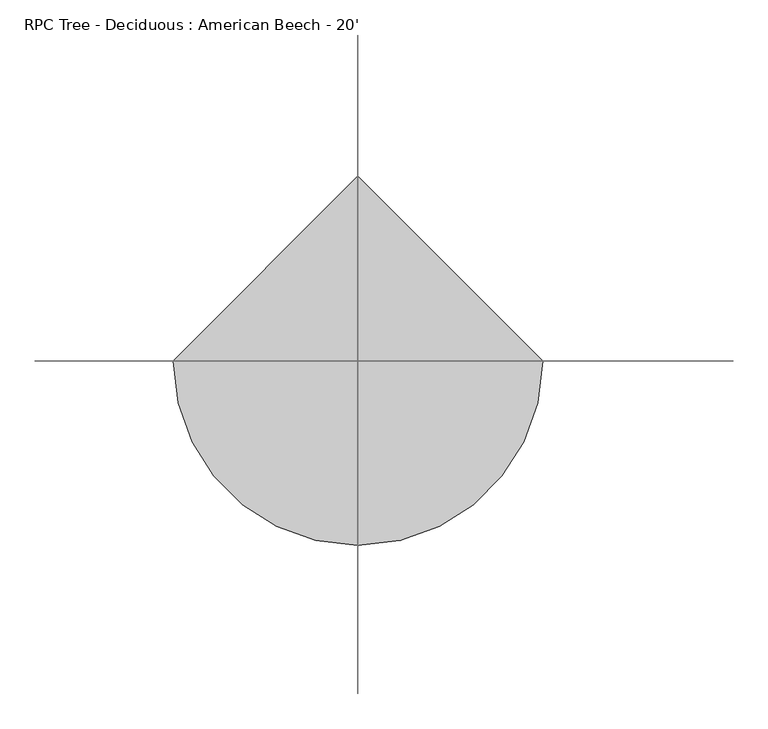
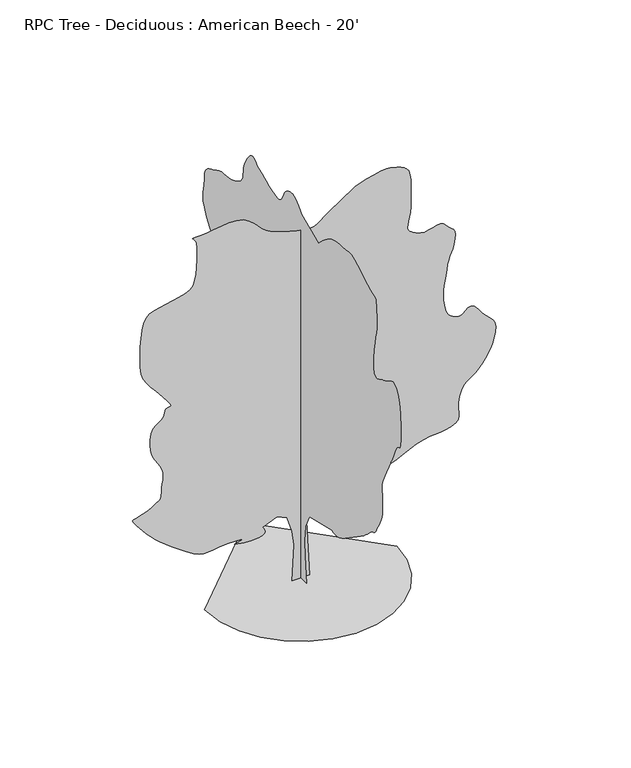
"""IFC4 building model written with IfcOpenShell, lengths in millimetres: geographic element geometry, RPC Tree - Deciduous : American Beech - 20'."""

from ifc_helpers import new_model, si_unit, origin, place, context, project, spatial, triangles, source, transform, mapped, element, save


def rpc_tree_deciduous_american_beech_20_b3c041c8(model_context):
    return source(origin(), model_context, "Body", "Tessellation", [
        triangles([(0.0009889, 136.856581, 0.0), (0.0009889, -149.8547884, 0.0), (0.0009889, -111.6264895, 420.510052), (0.0009889, -102.0697236, 659.4353302), (0.0009889, -121.1832463, 898.3606447), (0.0009889, -235.8678885, 1118.172373), (0.0009889, -818.8458761, 1261.5275036), (0.0009889, -849.9431059, 1249.7139805), (0.0009889, -883.2933231, 1240.7427258), (0.0009889, -921.1596891, 1237.4533916), (0.0009889, -965.7976622, 1242.6934788), (0.0009889, -1019.4603024, 1259.3000233), (0.0009889, -1084.4081549, 1290.1152935), (0.0009889, -1162.8992941, 1337.984174), (0.0009889, -1478.2811337, 1557.7959023), (0.0009889, -1522.8632961, 1589.1420994), (0.0009889, -1566.942437, 1618.9819931), (0.0009889, -1611.1893002, 1649.3249084), (0.0009889, -1656.2718681, 1682.1772636), (0.0009889, -1702.8579781, 1719.5406807), (0.0009889, -1751.6183739, 1763.4243393), (0.0009889, -1803.2210381, 1815.834803), (0.0009889, -1847.9404015, 1858.0191467), (0.0009889, -1878.9512993, 1877.1351311), (0.0009889, -1901.2702858, 1884.0440117), (0.0009889, -1919.9112991, 1889.616782), (0.0009889, -1939.8884228, 1904.7196392), (0.0009889, -1966.2180656, 1940.2161644), (0.0009889, -2003.916782, 2006.9774963), (0.0009889, -2044.9607883, 2083.2080177), (0.0009889, -2078.313549, 2145.2324295), (0.0009889, -2104.4754696, 2201.0692829), (0.0009889, -2123.9521877, 2258.7475937), (0.0009889, -2137.244109, 2326.2862038), (0.0009889, -2144.8488773, 2411.7141289), (0.0009889, -2147.2746014, 2523.0550072), (0.0009889, -2142.5373905, 2624.8889076), (0.0009889, -2132.7863869, 2688.2873634), (0.0009889, -2124.7040314, 2730.9338882), (0.0009889, -2124.9835201, 2770.583503), (0.0009889, -2140.3072941, 2824.9394875), (0.0009889, -2177.3659332, 2911.7568626), (0.0009889, -2242.84464, 3048.6883301), (0.0009889, -2308.7119858, 3181.9621719), (0.0009889, -2348.5011269, 3259.3812836), (0.0009889, -2371.2366577, 3301.215358), (0.0009889, -2385.9484051, 3327.6567673), (0.0009889, -2401.6632889, 3358.9496246), (0.0009889, -2427.4088104, 3415.3121727), (0.0009889, -2472.2118896, 3516.9885246), (0.0009889, -2522.8114174, 3609.6476944), (0.0009889, -2561.0332123, 3645.1568642), (0.0009889, -2588.5669968, 3652.9040657), (0.0009889, -2607.0580193, 3662.3273277), (0.0009889, -2618.2087921, 3702.8402618), (0.0009889, -2623.669796, 3803.856189), (0.0009889, -2625.117382, 3994.8390083), (0.0009889, -2615.3639076, 4210.713913), (0.0009889, -2589.2271309, 4371.4450905), (0.0009889, -2551.406765, 4483.8402649), (0.0009889, -2506.5400269, 4554.7824463), (0.0009889, -2459.3391289, 4591.1043571), (0.0009889, -2414.4802391, 4599.6895889), (0.0009889, -2376.641851, 4587.3705734), (0.0009889, -2343.8477772, 4566.9491455), (0.0009889, -2310.8862717, 4546.8576393), (0.0009889, -2277.5893215, 4527.4521378), (0.0009889, -2243.7921112, 4509.0116936), (0.0009889, -2209.3243023, 4491.9426773), (0.0009889, -2174.0232594, 4476.5250137), (0.0009889, -2137.7164639, 4463.1392029), (0.0009889, -2096.4236355, 4443.6572525), (0.0009889, -2049.6139927, 4418.4858238), (0.0009889, -2002.3013283, 4400.6805153), (0.0009889, -1959.504958, 4403.2713455), (0.0009889, -1926.2359131, 4439.313913), (0.0009889, -1907.5110386, 4521.8132378), (0.0009889, -1908.3467434, 4663.8246277), (0.0009889, -1923.6450829, 4819.4253044), (0.0009889, -1942.954224, 4940.7356323), (0.0009889, -1963.266647, 5037.9669067), (0.0009889, -1981.572361, 5121.3298416), (0.0009889, -1994.8642822, 5201.0354416), (0.0009889, -2000.1296585, 5287.2429703), (0.0009889, -1994.3614059, 5390.1634323), (0.0009889, -1986.3653824, 5488.9190323), (0.0009889, -1983.048143, 5559.911792), (0.0009889, -1978.5625156, 5609.3407516), (0.0009889, -1967.0562412, 5643.3764648), (0.0009889, -1942.6748806, 5668.2429703), (0.0009889, -1899.5709709, 5690.0869858), (0.0009889, -1831.8926891, 5715.1063889), (0.0009889, -1748.4408062, 5751.9616974), (0.0009889, -1662.820015, 5800.5261749), (0.0009889, -1576.3582867, 5853.7903656), (0.0009889, -1490.4020508, 5904.6919098), (0.0009889, -1406.2848015, 5946.2207703), (0.0009889, -1325.3426491, 5971.3924896), (0.0009889, -1248.913884, 5973.1447083), (0.0009889, -1174.2403896, 5963.3406555), (0.0009889, -1098.5636135, 5956.711409), (0.0009889, -1023.222064, 5950.5641098), (0.0009889, -949.5518515, 5942.2588028), (0.0009889, -878.8914843, 5929.1264648), (0.0009889, -812.5771454, 5908.4509827), (0.0009889, -751.9472706, 5877.5644958), (0.0009889, -697.9494038, 5841.2678741), (0.0009889, -649.9687569, 5805.9618896), (0.0009889, -607.0045916, 5771.4942261), (0.0009889, -568.0511189, 5737.7119858), (0.0009889, -532.1075644, 5704.4128555), (0.0009889, -498.1706097, 5671.4433563), (0.0009889, -465.2369368, 5638.6523346), (0.0009889, -16.056217, 5829.7871796), (0.0009889, 22.8405617, 5872.4339951), (0.0009889, 61.6537222, 5913.023378), (0.0009889, 100.2998553, 5949.3961578), (0.0009889, 138.6950317, 5979.5204819), (0.0009889, 176.7559443, 6001.2883392), (0.0009889, 214.3990318, 6012.5911377), (0.0009889, 251.5404602, 6011.3720261), (0.0009889, 287.2056524, 6002.4312927), (0.0009889, 320.3628219, 5991.305809), (0.0009889, 350.8454089, 5977.0055191), (0.0009889, 378.4856913, 5958.5397858), (0.0009889, 403.1160919, 5934.892392), (0.0009889, 424.5689612, 5905.047702), (0.0009889, 442.6817001, 5868.0144974), (0.0009889, 459.9562634, 5826.9425858), (0.0009889, 480.2407084, 5787.547316), (0.0009889, 505.3740581, 5752.6727005), (0.0009889, 537.1926464, 5725.138916), (0.0009889, 577.5380399, 5707.7911377), (0.0009889, 628.2491524, 5703.5239563), (0.0009889, 691.1650068, 5715.1063889), (0.0009889, 759.6790661, 5736.9754028), (0.0009889, 826.1890326, 5761.3593796), (0.0009889, 891.0251186, 5787.8263687), (0.0009889, 954.5251671, 5815.9694183), (0.0009889, 1017.0218611, 5845.3577408), (0.0009889, 1078.8506453, 5875.5832214), (0.0009889, 1140.3440575, 5906.2412338), (0.0009889, 1169.0715191, 5932.3524307), (0.0009889, 1198.1316639, 5955.3649796), (0.0009889, 1227.8624073, 5972.2052307), (0.0009889, 1258.5938164, 5979.7489563), (0.0009889, 1290.6664227, 5974.9230881), (0.0009889, 1324.4078224, 5954.6539764), (0.0009889, 1360.1557858, 5915.7918137), (0.0009889, 1395.1799561, 5868.217392), (0.0009889, 1426.1908539, 5822.9544571), (0.0009889, 1452.6880737, 5778.8856354), (0.0009889, 1474.1715008, 5734.7912338), (0.0009889, 1490.1379681, 5689.5538788), (0.0009889, 1500.0845993, 5641.9538773), (0.0009889, 1503.510989, 5590.8494385), (0.0009889, 1507.2168674, 5539.3380478), (0.0009889, 1519.1142517, 5491.1793594), (0.0009889, 1540.3740005, 5446.1704788), (0.0009889, 1572.1672634, 5404.1846695), (0.0009889, 1615.6596668, 5365.0428726), (0.0009889, 1672.0274471, 5328.5689362), (0.0009889, 1742.4363762, 5294.5832199), (0.0009889, 1817.5288857, 5269.1836075), (0.0009889, 1887.9378147, 5255.1373718), (0.0009889, 1954.8363476, 5247.4407486), (0.0009889, 2019.3956337, 5241.0911362), (0.0009889, 2082.7839157, 5231.0580276), (0.0009889, 2146.1721977, 5212.3382401), (0.0009889, 2210.7313385, 5179.9024292), (0.0009889, 2276.3498623, 5145.3580261), (0.0009889, 2340.1267834, 5118.8404587), (0.0009889, 2399.0573433, 5093.1356323), (0.0009889, 2450.1315514, 5061.106192), (0.0009889, 2490.3372368, 5015.5136261), (0.0009889, 2516.667025, 4949.193837), (0.0009889, 2526.1132507, 4854.9597633), (0.0009889, 2532.46577, 4758.008123), (0.0009889, 2546.5044479, 4681.9348595), (0.0009889, 2560.7285797, 4617.2411339), (0.0009889, 2567.5865913, 4554.3760757), (0.0009889, 2559.5600464, 4483.8402649), (0.0009889, 2529.1232414, 4396.0578323), (0.0009889, 2468.7702393, 4281.5543564), (0.0009889, 2394.0992157, 4166.6192207), (0.0009889, 2326.6139454, 4078.2525215), (0.0009889, 2267.6553349, 4007.9707649), (0.0009889, 2218.5596397, 3947.1884285), (0.0009889, 2180.6679119, 3887.4223091), (0.0009889, 2155.3111748, 3820.1377533), (0.0009889, 2143.8328056, 3736.8001076), (0.0009889, 2149.4334812, 3646.0204742), (0.0009889, 2171.0820145, 3561.7686401), (0.0009889, 2203.7667927, 3483.5112076), (0.0009889, 2242.4687908, 3410.790937), (0.0009889, 2282.1714546, 3343.1000107), (0.0009889, 2317.8662235, 3279.9047401), (0.0009889, 2344.5311657, 3220.7225967), (0.0009889, 2370.3577869, 3180.6921913), (0.0009889, 2402.5396889, 3164.8934464), (0.0009889, 2434.5538685, 3157.7813805), (0.0009889, 2459.8827003, 3143.8113029), (0.0009889, 2472.0037628, 3107.4638123), (0.0009889, 2464.3963783, 3033.1433487), (0.0009889, 2430.5432121, 2905.3305107), (0.0009889, 2383.9011463, 2761.3378464), (0.0009889, 2340.6017544, 2643.9136185), (0.0009889, 2298.1379219, 2545.7425758), (0.0009889, 2254.0028252, 2459.415287), (0.0009889, 2205.6894951, 2377.6095245), (0.0009889, 2150.6857304, 2292.9614937), (0.0009889, 2086.4897942, 2198.1177189), (0.0009889, 2022.098085, 2102.5196297), (0.0009889, 1968.0723129, 2019.6267242), (0.0009889, 1924.2446102, 1948.102747), (0.0009889, 1890.4447838, 1886.6067913), (0.0009889, 1866.5103436, 1833.8078339), (0.0009889, 1852.2735672, 1788.3620613), (0.0009889, 1847.564407, 1748.9361248), (0.0009889, 1851.5776794, 1721.8800728), (0.0009889, 1860.940044, 1709.2029396), (0.0009889, 1871.6386642, 1703.0459026), (0.0009889, 1879.6624477, 1695.5504299), (0.0009889, 1881.0010288, 1678.8600243), (0.0009889, 1871.6386642, 1645.1186245), (0.0009889, 1847.564407, 1586.4675533), (0.0009889, 1827.5314728, 1524.5828133), (0.0009889, 1825.3850922, 1482.2587978), (0.0009889, 1829.7590984, 1453.3104195), (0.0009889, 1829.2865982, 1431.547649), (0.0009889, 1812.5961926, 1410.7907764), (0.0009889, 1768.3214241, 1384.8497726), (0.0009889, 1685.0958355, 1347.5421661), (0.0009889, 1594.399918, 1309.4244347), (0.0009889, 1528.281134, 1282.5080544), (0.0009889, 1476.2059696, 1262.7823689), (0.0009889, 1427.6412014, 1246.2316349), (0.0009889, 1372.05317, 1228.8453415), (0.0009889, 1298.9138844, 1206.6102161), (0.0009889, 1197.6871416, 1175.5154572), (0.0009889, 1096.069289, 1145.7009253), (0.0009889, 1022.5387482, 1127.7557997), (0.0009889, 967.7331545, 1118.3400227), (0.0009889, 922.2874546, 1114.10329), (0.0009889, 876.8442255, 1111.7080873), (0.0009889, 822.0360884, 1107.806654), (0.0009889, 748.5055475, 1099.0588594), (0.0009889, 662.4935011, 1085.0990284), (0.0009889, 576.4788749, 1068.1292793), (0.0009889, 490.4667558, 1048.6551046), (0.0009889, 404.4521296, 1027.1717503), (0.0009889, 318.4400468, 1004.1847086), (0.0009889, 232.4266923, 980.1943851), (0.0009889, 146.4133378, 955.7037289), (136.1842383, 0.0003154, 0.014068), (-131.4120823, 0.0003154, 0.014068), (-102.7410489, 0.0002819, 563.8778998), (-131.4120823, 0.0002692, 793.2477293), (-207.8684348, 0.0002549, 1032.1729712), (-360.7819027, 0.0002501, 1108.6296415), (-580.5936673, 0.0002549, 1013.0594576), (-562.704425, 0.0002564, 988.5662579), (-548.0765751, 0.000258, 964.5784779), (-539.9688578, 0.0002596, 941.5914362), (-541.6401947, 0.0002612, 920.1080818), (-556.3518694, 0.0002628, 900.6313637), (-587.3627672, 0.0002628, 883.6641581), (-637.9342443, 0.0002644, 869.704327), (-697.421093, 0.0002644, 860.4815615), (-753.4001616, 0.0002644, 856.775683), (-806.4506298, 0.0002644, 857.667271), (-857.1617786, 0.0002644, 862.2366869), (-906.117802, 0.0002644, 869.5645826), (-953.9028214, 0.0002628, 878.731465), (-1001.1011759, 0.0002628, 888.8178406), (-953.2881786, 0.0002628, 900.9945683), (-913.501581, 0.0002612, 912.5008427), (-889.7601522, 0.0002612, 922.6710068), (-890.0954515, 0.0002596, 930.8345346), (-922.5287189, 0.0002596, 936.3235165), (-995.0838833, 0.0002596, 938.4698244), (-1115.7848007, 0.0002596, 936.6028599), (-1242.9524746, 0.0002612, 927.8271601), (-1337.3542706, 0.0002612, 914.3677345), (-1410.6891838, 0.0002612, 903.2500992), (-1474.6617325, 0.0002612, 901.4949738), (-1540.9759987, 0.0002612, 916.12286), (-1621.3340298, 0.0002596, 954.1568756), (-1727.4351116, 0.0002549, 1022.614979), (-1845.0726986, 0.0002501, 1105.8432564), (-1952.34711, 0.0002453, 1184.0549795), (-2049.4209812, 0.0002405, 1258.0858532), (-2136.46436, 0.0002373, 1328.7765965), (-2213.6472942, 0.0002326, 1396.9554291), (-2281.1300938, 0.0002278, 1463.4653229), (-2339.0852772, 0.0002246, 1529.1396572), (-2391.8031349, 0.0002214, 1592.6651402), (-2441.3431343, 0.0002166, 1651.1791557), (-2484.5309052, 0.0002134, 1703.170459), (-2518.1884438, 0.0002118, 1747.1378334), (-2539.1409439, 0.0002103, 1781.577737), (-2544.218541, 0.0002087, 1804.9838665), (-2530.2254997, 0.0002071, 1815.8500637), (-2498.742247, 0.0002071, 1822.7308937), (-2456.2227493, 0.0002071, 1834.628278), (-2406.8475655, 0.0002055, 1850.7065117), (-2354.8003063, 0.0002039, 1870.1272739), (-2304.2568798, 0.0002023, 1892.0551506), (-2259.3978447, 0.0002023, 1915.6542915), (-2224.401725, 0.0002007, 1940.091608), (-2196.9849392, 0.0001991, 1958.6464348), (-2172.4078056, 0.0001991, 1969.1798035), (-2151.1759621, 0.0001975, 1977.7066086), (-2133.7896687, 0.0001975, 1990.2439247), (-2120.7518017, 0.0001959, 2012.8144947), (-2112.5602959, 0.0001927, 2051.4326317), (-2109.7180275, 0.0001895, 2112.118317), (-2105.7607109, 0.0001864, 2181.0514641), (-2096.7894562, 0.0001816, 2242.2935108), (-2087.1476028, 0.0001784, 2298.6891964), (-2081.1861935, 0.0001752, 2353.0781731), (-2083.2487129, 0.000172, 2408.3028545), (-2097.6809715, 0.0001688, 2467.2028931), (-2128.8315411, 0.0001641, 2532.6259346), (-2168.3971493, 0.0001609, 2596.7202782), (-2204.2849297, 0.0001577, 2653.2860115), (-2235.1560104, 0.0001545, 2707.6675758), (-2259.6771881, 0.0001513, 2765.2239464), (-2276.5047947, 0.0001465, 2831.3149704), (-2284.3076614, 0.0001418, 2911.2740433), (-2281.7447365, 0.000137, 3010.4865921), (-2264.5514545, 0.0001306, 3102.7902603), (-2233.1494469, 0.0001274, 3164.9948936), (-2193.2231049, 0.0001242, 3206.8286774), (-2150.4520237, 0.0001226, 3237.9439293), (-2110.525827, 0.0001211, 3268.0682533), (-2079.123674, 0.0001179, 3306.8795471), (-2061.9330082, 0.0001147, 3364.0804161), (-2043.9599773, 0.0001131, 3413.0262657), (-2014.1200836, 0.0001115, 3431.3396828), (-1983.9422745, 0.0001115, 3435.3019409), (-1964.9684326, 0.0001099, 3441.0931572), (-1968.7301216, 0.0001099, 3464.9437363), (-2006.7641373, 0.0001051, 3523.0843735), (-2090.6020432, 9.88e-05, 3631.6948952), (-2191.4121689, 9.24e-05, 3753.7165169), (-2273.3296978, 8.6e-05, 3849.6778107), (-2337.3582024, 8.12e-05, 3932.1009773), (-2384.5031445, 7.65e-05, 4013.5079269), (-2415.7654804, 7.17e-05, 4106.47202), (-2432.1484921, 6.37e-05, 4223.4898773), (-2434.6554611, 5.42e-05, 4377.1345688), (-2429.5297565, 4.46e-05, 4541.5998207), (-2420.5585018, 3.66e-05, 4683.0016548), (-2405.0643894, 3.03e-05, 4801.6705742), (-2380.3781055, 2.39e-05, 4897.9365005), (-2343.822488, 1.91e-05, 4972.1558075), (-2292.720084, 1.59e-05, 5024.6066757), (-2224.401725, 1.43e-05, 5055.6710587), (-2138.4149677, 1.27e-05, 5074.7972168), (-2040.8941761, 1.27e-05, 5092.7292618), (-1939.0274288, 1.11e-05, 5111.8554199), (-1840.0028046, 9.6e-06, 5134.487178), (-1751.0088181, 8e-06, 5162.9604401), (-1679.2334026, 6.4e-06, 5199.612854), (-1631.8649277, 3.2e-06, 5246.8314835), (-1604.1128426, -1.6e-06, 5316.4272354), (-1585.3905842, -6.4e-06, 5411.6010773), (-1574.1890877, -1.27e-05, 5521.6594757), (-1569.0075726, -2.07e-05, 5635.9088974), (-1568.336974, -2.71e-05, 5743.6302292), (-1570.6788368, -3.19e-05, 5834.1305191), (-1574.524387, -3.5e-05, 5896.690654), (-1585.918895, -3.82e-05, 5936.1626633), (-1606.0102558, -3.98e-05, 5965.4230865), (-1625.9315689, -4.14e-05, 5985.9718323), (-1636.825526, -4.14e-05, 5999.3576431), (-1629.8329296, -4.3e-05, 6007.0286865), (-1596.0890591, -4.3e-05, 6010.559285), (-1526.7393677, -4.3e-05, 6011.3976059), (-1428.7715103, -4.3e-05, 6017.8233765), (-1318.7690678, -4.46e-05, 6032.4538788), (-1202.2439129, -4.46e-05, 6048.2529144), (-1084.7180197, -4.46e-05, 6058.184285), (-971.7057318, -4.46e-05, 6055.263533), (-868.7238636, -4.46e-05, 6032.4538788), (-781.2893749, -4.14e-05, 5982.7208679), (-714.8937183, -3.66e-05, 5922.6245361), (-665.5465851, -3.34e-05, 5871.6974121), (-624.5610781, -3.19e-05, 5827.4756927), (-583.2403444, -2.87e-05, 5787.445578), (-532.8924365, -2.71e-05, 5749.0915237), (-464.8228995, -2.39e-05, 5709.8735687), (-370.3373878, -2.23e-05, 5667.3284912), (-260.8632923, -1.91e-05, 5627.3745346), (-155.7366604, -1.75e-05, 5596.9449966), (-58.1322665, -1.59e-05, 5575.0504028), (28.7726351, -1.59e-05, 5560.6739548), (101.8020074, -1.59e-05, 5552.8255966), (157.7788323, -1.43e-05, 5550.4629501), (193.5270681, -1.59e-05, 5552.6477005), (219.2725352, -1.59e-05, 5560.6233765), (247.3583572, -1.59e-05, 5575.4311935), (277.7847885, -1.75e-05, 5595.7770447), (310.5508118, -1.91e-05, 5620.2877579), (345.6587342, -2.07e-05, 5647.6692261), (383.1059761, -2.23e-05, 5676.5232788), (422.8950809, -2.39e-05, 5705.555809), (805.1781057, -3.98e-05, 5963.5947098), (830.3647951, -3.98e-05, 5972.992392), (896.679134, -4.14e-05, 5996.5892075), (990.2426817, -4.3e-05, 6027.5518524), (1097.1817938, -4.62e-05, 6058.9970261), (1203.6180296, -4.62e-05, 6084.1175858), (1295.67789, -4.78e-05, 6096.0046509), (1359.4853325, -4.78e-05, 6087.8516602), (1407.4912685, -4.62e-05, 6070.6556168), (1459.1777939, -4.46e-05, 6056.8128571), (1511.1996185, -4.46e-05, 6041.4457718), (1560.2089817, -4.3e-05, 6019.7540726), (1602.8682964, -4.14e-05, 5986.835733), (1635.8299473, -3.82e-05, 5937.8898834), (1655.7537312, -3.34e-05, 5868.0394958), (1665.3091072, -2.87e-05, 5789.7820633), (1670.1859898, -2.55e-05, 5717.2399796), (1671.5500053, -2.07e-05, 5647.8471222), (1670.5746288, -1.75e-05, 5579.1396881), (1668.4282482, -1.27e-05, 5508.6038773), (1666.2844837, -8e-06, 5433.699147), (1665.3091072, -3.2e-06, 5351.9622757), (1660.2367424, 1.6e-06, 5270.5806152), (1648.1463467, 6.4e-06, 5198.4187408), (1633.7114719, 9.6e-06, 5135.2743393), (1621.6186054, 1.27e-05, 5081.0200928), (1616.5487114, 1.59e-05, 5035.4269455), (1623.1807194, 1.75e-05, 4998.368161), (1646.1955936, 1.91e-05, 4969.6664246), (1678.4054008, 2.07e-05, 4946.8317719), (1709.6119263, 2.23e-05, 4927.324823), (1739.9826015, 2.23e-05, 4910.992099), (1769.6829689, 2.39e-05, 4897.6824463), (1798.8852562, 2.39e-05, 4887.1923889), (1827.7499187, 2.55e-05, 4879.3946091), (1856.4493298, 2.55e-05, 4874.0862122), (1893.0609032, 2.55e-05, 4877.1087021), (1942.2125542, 2.39e-05, 4889.9864044), (1998.8851124, 2.39e-05, 4906.1918106), (2058.0671104, 2.23e-05, 4919.2474091), (2114.7396687, 2.23e-05, 4922.5745316), (2163.8911743, 2.39e-05, 4909.6968292), (2200.5028931, 2.55e-05, 4874.0862122), (2230.4850746, 2.71e-05, 4834.208123), (2261.3003448, 2.87e-05, 4807.6649757), (2290.2766285, 3.03e-05, 4786.8368866), (2314.7419956, 3.19e-05, 4763.9769447), (2332.0165226, 3.34e-05, 4731.4396866), (2339.4282795, 3.66e-05, 4681.5031998), (2334.3025749, 4.14e-05, 4606.4970222), (2319.8956055, 4.62e-05, 4526.9440292), (2302.1485783, 4.94e-05, 4463.951944), (2282.3925167, 5.26e-05, 4410.6627548), (2261.9683273, 5.57e-05, 4360.1928703), (2242.2147366, 5.89e-05, 4305.7098587), (2224.4652386, 6.37e-05, 4240.3809975), (2210.0608852, 6.85e-05, 4157.3229858), (2196.9087811, 7.33e-05, 4068.4481781), (2183.2562714, 7.8e-05, 3988.0827347), (2170.9397266, 8.28e-05, 3913.0762665), (2161.8007496, 8.76e-05, 3840.2289688), (2157.6783268, 9.08e-05, 3766.3913246), (2160.4088287, 9.56e-05, 3688.3876556), (2171.831242, 0.0001003, 3603.0181572), (2189.9719952, 0.0001051, 3525.0147789), (2211.6203831, 0.0001083, 3468.2711494), (2236.7791672, 0.0001115, 3428.240744), (2265.4506729, 0.0001131, 3400.402327), (2297.6324295, 0.0001147, 3380.2602425), (2333.3271984, 0.0001147, 3363.2673843), (2372.5296021, 0.0001163, 3344.9795471), (2412.5675652, 0.0001163, 3342.4901642), (2451.7724396, 0.0001147, 3366.0869797), (2491.642971, 0.0001131, 3400.8848557), (2533.6901138, 0.0001115, 3432.0253967), (2579.4227875, 0.0001099, 3444.5728867), (2630.3246223, 0.0001115, 3423.7195084), (2687.906282, 0.0001163, 3354.5298363), (2749.8568611, 0.0001211, 3269.9730789), (2810.1313797, 0.0001242, 3206.9557045), (2864.6905495, 0.0001274, 3156.6637161), (2909.5976921, 0.0001306, 3110.2325386), (2940.7635223, 0.0001338, 3058.7720169), (2954.2254913, 0.000137, 2993.4178665), (2945.9451828, 0.0001434, 2905.3557999), (2924.1520363, 0.0001481, 2810.6139084), (2899.209082, 0.0001529, 2729.079641), (2870.2277115, 0.0001577, 2657.6040619), (2836.3948929, 0.0001609, 2592.9612053), (2796.8723053, 0.0001641, 2531.9858574), (2750.8474983, 0.0001688, 2471.5235596), (2697.4568619, 0.000172, 2408.3842449), (2642.4404526, 0.0001752, 2354.2186558), (2591.9196991, 0.0001784, 2316.7713776), (2545.7425758, 0.00018, 2287.0127289), (2503.7637428, 0.0001816, 2255.9181152), (2465.7858284, 0.0001832, 2214.4575645), (2431.6531734, 0.000188, 2153.606773), (2401.2011078, 0.0001927, 2064.3332977), (2384.7901909, 0.0001991, 1965.7532684), (2385.7654221, 0.0002039, 1881.8849865), (2393.4261463, 0.0002071, 1811.0570423), (2397.0760689, 0.0002118, 1751.5981716), (2386.0143894, 0.000215, 1701.8343487), (2349.5424877, 0.0002166, 1660.0945999), (2276.9594181, 0.0002182, 1624.7096958), (2189.7484623, 0.0002198, 1601.1638947), (2111.7322941, 0.0002214, 1590.8261536), (2035.7202187, 0.0002214, 1585.8401207), (1954.5264828, 0.0002214, 1578.3445026), (1860.9630077, 0.000223, 1560.4858543), (1747.8389534, 0.0002246, 1524.4025917), (1607.9660957, 0.0002294, 1462.2385082), (1455.667543, 0.0002326, 1390.7425816), (1311.7282185, 0.0002357, 1331.4512878), (1178.6524023, 0.0002389, 1283.6941738), (1058.9547667, 0.0002421, 1246.8031116), (955.1372663, 0.0002437, 1220.1102642), (869.7094139, 0.0002437, 1202.9449602), (805.1781057, 0.0002453, 1194.641688), (403.7815673, 0.0002453, 1185.0862392), (107.513205, 0.0002485, 1137.3011473), (88.3996914, 0.0002628, 879.2597757), (-1453.7574852, 0.0, 0.0120292), (-1415.3246567, -333.1060121, 0.0120292), (-1305.8708725, -639.0085974, 0.0120292), (-1134.1566444, -908.9473532, 0.0120292), (-908.9473532, -1134.1566444, 0.0120292), (-639.0085974, -1305.8708725, 0.0120292), (-333.1060121, -1415.3246567, 0.0120292), (6.35e-05, -1453.7574852, 0.0120292), (333.1060121, -1415.3246567, 0.0120292), (639.0085974, -1305.8708725, 0.0120292), (908.9473532, -1134.1566444, 0.0120292), (1134.1566444, -908.9473532, 0.0120292), (1305.8708725, -639.0085974, 0.0120292), (1415.3246567, -333.1060121, 0.0120292), (1453.7574852, 0.0001274, 0.0120292), (-0.0001906, 1453.7574852, 0.0120292)], [[1, 2, 3], [254, 1, 3], [254, 3, 4], [254, 4, 5], [254, 5, 6], [53, 54, 55], [52, 53, 55], [201, 202, 203], [201, 203, 204], [200, 201, 204], [222, 223, 224], [52, 55, 56], [200, 204, 205], [199, 200, 205], [253, 254, 6], [221, 222, 224], [221, 224, 225], [229, 230, 231], [229, 231, 232], [228, 229, 232], [228, 232, 233], [227, 228, 233], [252, 253, 6], [221, 225, 226], [220, 221, 226], [199, 205, 206], [198, 199, 206], [62, 63, 64], [61, 62, 64], [61, 64, 65], [60, 61, 65], [60, 65, 66], [59, 60, 66], [59, 66, 67], [59, 67, 68], [58, 59, 68], [58, 68, 69], [58, 69, 70], [57, 58, 70], [57, 70, 71], [57, 71, 72], [57, 72, 73], [57, 73, 74], [56, 57, 74], [52, 56, 74], [51, 52, 74], [50, 51, 74], [50, 74, 75], [49, 50, 75], [48, 49, 75], [47, 48, 75], [46, 47, 75], [45, 46, 75], [44, 45, 75], [43, 44, 75], [42, 43, 75], [42, 75, 76], [41, 42, 76], [227, 233, 234], [226, 227, 234], [220, 226, 234], [219, 220, 234], [219, 234, 235], [219, 235, 236], [219, 236, 237], [218, 219, 237], [218, 237, 238], [218, 238, 239], [218, 239, 240], [217, 218, 240], [217, 240, 241], [217, 241, 242], [217, 242, 243], [217, 243, 244], [217, 244, 245], [217, 245, 246], [216, 217, 246], [216, 246, 247], [215, 216, 247], [215, 247, 248], [251, 252, 6], [88, 89, 90], [88, 90, 91], [87, 88, 91], [87, 91, 92], [86, 87, 92], [86, 92, 93], [85, 86, 93], [84, 85, 93], [84, 93, 94], [83, 84, 94], [82, 83, 94], [81, 82, 94], [81, 94, 95], [80, 81, 95], [80, 95, 96], [80, 96, 97], [80, 97, 98], [80, 98, 99], [80, 99, 100], [80, 100, 101], [80, 101, 102], [80, 102, 103], [80, 103, 104], [80, 104, 105], [80, 105, 106], [80, 106, 107], [80, 107, 108], [80, 108, 109], [80, 109, 110], [80, 110, 111], [80, 111, 112], [79, 80, 112], [79, 112, 113], [78, 79, 113], [77, 78, 113], [76, 77, 113], [41, 76, 113], [40, 41, 113], [40, 113, 114], [39, 40, 114], [198, 206, 207], [197, 198, 207], [196, 197, 207], [196, 207, 208], [195, 196, 208], [195, 208, 209], [195, 209, 210], [195, 210, 211], [194, 195, 211], [194, 211, 212], [194, 212, 213], [193, 194, 213], [193, 213, 214], [214, 215, 248], [193, 214, 248], [193, 248, 249], [192, 193, 249], [192, 249, 250], [192, 250, 251], [192, 251, 6], [192, 6, 7], [191, 192, 7], [190, 191, 7], [189, 190, 7], [38, 39, 114], [37, 38, 114], [36, 37, 114], [35, 36, 114], [34, 35, 114], [33, 34, 114], [32, 33, 114], [31, 32, 114], [30, 31, 114], [29, 30, 114], [28, 29, 114], [27, 28, 114], [26, 27, 114], [25, 26, 114], [24, 25, 114], [23, 24, 114], [22, 23, 114], [21, 22, 114], [20, 21, 114], [19, 20, 114], [18, 19, 114], [17, 18, 114], [16, 17, 114], [15, 16, 114], [14, 15, 114], [13, 14, 114], [12, 13, 114], [11, 12, 114], [10, 11, 114], [9, 10, 114], [8, 9, 114], [7, 8, 114], [189, 7, 114], [188, 189, 114], [188, 114, 115], [188, 115, 116], [188, 116, 117], [188, 117, 118], [188, 118, 119], [188, 119, 120], [188, 120, 121], [146, 147, 148], [145, 146, 148], [144, 145, 148], [144, 148, 149], [143, 144, 149], [143, 149, 150], [142, 143, 150], [142, 150, 151], [142, 151, 152], [141, 142, 152], [141, 152, 153], [141, 153, 154], [141, 154, 155], [141, 155, 156], [140, 141, 156], [140, 156, 157], [139, 140, 157], [138, 139, 157], [138, 157, 158], [137, 138, 158], [137, 158, 159], [136, 137, 159], [135, 136, 159], [135, 159, 160], [134, 135, 160], [134, 160, 161], [174, 175, 176], [173, 174, 176], [173, 176, 177], [172, 173, 177], [171, 172, 177], [171, 177, 178], [170, 171, 178], [170, 178, 179], [169, 170, 179], [168, 169, 179], [167, 168, 179], [166, 167, 179], [165, 166, 179], [165, 179, 180], [165, 180, 181], [165, 181, 182], [165, 182, 183], [165, 183, 184], [165, 184, 185], [165, 185, 186], [165, 186, 187], [164, 165, 187], [164, 187, 188], [163, 164, 188], [162, 163, 188], [161, 162, 188], [134, 161, 188], [133, 134, 188], [132, 133, 188], [125, 126, 127], [124, 125, 127], [124, 127, 128], [123, 124, 128], [122, 123, 128], [121, 122, 128], [121, 128, 129], [121, 129, 130], [121, 130, 131], [188, 121, 131], [132, 188, 131], [274, 275, 276], [531, 255, 256], [531, 256, 257], [531, 257, 258], [531, 258, 259], [530, 531, 259], [376, 377, 378], [376, 378, 379], [375, 376, 379], [273, 274, 276], [273, 276, 277], [375, 379, 380], [374, 375, 380], [273, 277, 278], [272, 273, 278], [301, 302, 303], [301, 303, 304], [300, 301, 304], [300, 304, 305], [299, 300, 305], [299, 305, 306], [298, 299, 306], [298, 306, 307], [297, 298, 307], [297, 307, 308], [271, 272, 278], [296, 297, 308], [296, 308, 309], [373, 374, 380], [373, 380, 381], [372, 373, 381], [295, 296, 309], [295, 309, 310], [294, 295, 310], [294, 310, 311], [294, 311, 312], [294, 312, 313], [293, 294, 313], [293, 313, 314], [292, 293, 314], [271, 278, 279], [291, 292, 314], [530, 259, 260], [372, 381, 382], [371, 372, 382], [291, 314, 315], [290, 291, 315], [371, 382, 383], [370, 371, 383], [370, 383, 384], [369, 370, 384], [369, 384, 385], [369, 385, 386], [369, 386, 387], [369, 387, 388], [369, 388, 389], [369, 389, 390], [368, 369, 390], [368, 390, 391], [367, 368, 391], [367, 391, 392], [367, 392, 393], [366, 367, 393], [366, 393, 394], [270, 271, 279], [366, 394, 395], [338, 339, 340], [338, 340, 341], [289, 290, 315], [483, 484, 485], [483, 485, 486], [482, 483, 486], [481, 482, 486], [481, 486, 487], [480, 481, 487], [288, 289, 315], [287, 288, 315], [286, 287, 315], [285, 286, 315], [284, 285, 315], [283, 284, 315], [282, 283, 315], [282, 315, 316], [281, 282, 316], [281, 316, 317], [281, 317, 318], [281, 318, 319], [281, 319, 320], [280, 281, 320], [280, 320, 321], [279, 280, 321], [279, 321, 322], [480, 487, 488], [264, 265, 266], [263, 264, 266], [263, 266, 267], [262, 263, 267], [262, 267, 268], [261, 262, 268], [261, 268, 269], [261, 269, 270], [261, 270, 279], [261, 279, 322], [260, 261, 322], [530, 260, 322], [530, 322, 323], [529, 530, 323], [529, 323, 324], [366, 395, 396], [365, 366, 396], [337, 338, 341], [337, 341, 342], [529, 324, 325], [528, 529, 325], [527, 528, 325], [526, 527, 325], [525, 526, 325], [524, 525, 325], [523, 524, 325], [522, 523, 325], [521, 522, 325], [521, 325, 326], [521, 326, 327], [521, 327, 328], [521, 328, 329], [521, 329, 330], [521, 330, 331], [521, 331, 332], [521, 332, 333], [521, 333, 334], [521, 334, 335], [521, 335, 336], [521, 336, 337], [521, 337, 342], [520, 521, 342], [520, 342, 343], [519, 520, 343], [518, 519, 343], [518, 343, 344], [517, 518, 344], [449, 450, 451], [448, 449, 451], [448, 451, 452], [447, 448, 452], [446, 447, 452], [446, 452, 453], [516, 517, 344], [515, 516, 344], [514, 515, 344], [513, 514, 344], [512, 513, 344], [511, 512, 344], [510, 511, 344], [509, 510, 344], [508, 509, 344], [507, 508, 344], [506, 507, 344], [505, 506, 344], [504, 505, 344], [503, 504, 344], [502, 503, 344], [501, 502, 344], [500, 501, 344], [499, 500, 344], [498, 499, 344], [497, 498, 344], [496, 497, 344], [495, 496, 344], [494, 495, 344], [493, 494, 344], [492, 493, 344], [491, 492, 344], [490, 491, 344], [489, 490, 344], [488, 489, 344], [480, 488, 344], [479, 480, 344], [478, 479, 344], [477, 478, 344], [476, 477, 344], [475, 476, 344], [474, 475, 344], [473, 474, 344], [472, 473, 344], [471, 472, 344], [470, 471, 344], [469, 470, 344], [468, 469, 344], [467, 468, 344], [466, 467, 344], [465, 466, 344], [464, 465, 344], [463, 464, 344], [463, 344, 345], [462, 463, 345], [462, 345, 346], [461, 462, 346], [460, 461, 346], [459, 460, 346], [458, 459, 346], [457, 458, 346], [456, 457, 346], [455, 456, 346], [454, 455, 346], [453, 454, 346], [446, 453, 346], [445, 446, 346], [444, 445, 346], [443, 444, 346], [442, 443, 346], [441, 442, 346], [440, 441, 346], [439, 440, 346], [438, 439, 346], [437, 438, 346], [436, 437, 346], [435, 436, 346], [435, 346, 347], [435, 347, 348], [435, 348, 349], [435, 349, 350], [435, 350, 351], [435, 351, 352], [435, 352, 353], [435, 353, 354], [435, 354, 355], [435, 355, 356], [435, 356, 357], [435, 357, 358], [435, 358, 359], [435, 359, 360], [435, 360, 361], [435, 361, 362], [435, 362, 363], [435, 363, 364], [435, 364, 365], [435, 365, 396], [435, 396, 397], [435, 397, 398], [435, 398, 399], [435, 399, 400], [435, 400, 401], [435, 401, 402], [435, 402, 403], [435, 403, 404], [435, 404, 405], [435, 405, 406], [435, 406, 407], [435, 407, 408], [435, 408, 409], [434, 435, 409], [433, 434, 409], [432, 433, 409], [431, 432, 409], [430, 431, 409], [429, 430, 409], [429, 409, 410], [429, 410, 411], [429, 411, 412], [428, 429, 412], [428, 412, 413], [427, 428, 413], [426, 427, 413], [426, 413, 414], [425, 426, 414], [425, 414, 415], [425, 415, 416], [425, 416, 417], [424, 425, 417], [424, 417, 418], [423, 424, 418], [423, 418, 419], [422, 423, 419], [422, 419, 420], [421, 422, 420], [546, 547, 532], [545, 546, 532], [545, 532, 533], [544, 545, 533], [544, 533, 534], [544, 534, 535], [543, 544, 535], [542, 543, 535], [542, 535, 536], [542, 536, 537], [542, 537, 538], [542, 538, 539], [542, 539, 540], [542, 540, 541]], closed=False),
    ])


if __name__ == "__main__":
    model = new_model("IFC4")
    model_context = context("Model", 3, world=origin())
    ifc_project = project(units=[si_unit("LENGTHUNIT", "METRE", prefix="MILLI")], contexts=[model_context])
    site = spatial("IfcSite", under=ifc_project)
    building = spatial("IfcBuilding", under=site)
    placement = place(None, origin())
    rpc_tree_deciduous_american_beech_20_shape = rpc_tree_deciduous_american_beech_20_b3c041c8(model_context)
    element("IfcGeographicElement", 1, ObjectType="RPC Tree - Deciduous : American Beech - 20'", at=placement, inside=building, context=model_context, shape_type="MappedRepresentation", body=[
        mapped(rpc_tree_deciduous_american_beech_20_shape, transform((0.0, 0.0, 0.0), x_axis=(1.0, 0.0, 0.0), y_axis=(0.0, 1.0, 0.0), z_axis=(0.0, 0.0, 1.0))),
    ])
    save(model, "model.ifc")

# Revit data of these elements
# Type "RPC Tree - Deciduous : American Beech - 20'"
#   built-in parameter 1005198 = "{2, 15},{39, RPC-16-G1GQ-43Q0-7NP3-0000-ST1L-LVER-AU},{1, 0},{1, 0},{2, 35},{1, 8},{5, Color},{1, 0},{1, 0},{3, 0.8},{3, 0.8},{3, 0.8},{1, 8},{7, BBoxMin},{1, 0},{1, 0},{1, 0},{1, 0},{1, 0},{1, 8},{7, BBoxMax},{1, 0},{1, 0},{1, 0},{1, 0},{1, 0},{2, 11},{9, RPCTypeId},{1, 0},{1, 0},{39, RPC-16-G1GQ-43Q0-7NP3-0000-ST1L-LVER-AU},{1, 6},{14, RPCPlantHeight},{1, 0},{1, 0},{2, 20},{2, 11},{7, keyword},{1, 0},{1, 0},{126, :Geometry:RPC:American Beech:Fagus grandifolia:The beech genus comprises about 10 species; American beech is native to Canada.},{2, 11},{8, category},{1, 0},{1, 0},{16, :Trees [General]},{2, 11},{12, LocalizedUID},{1, 0},{1, 0},{14, American Beech},{2, 14},{6, Height},{1, 0},{1, 0},{2, 20},{1, 2},{16, Cast Reflections},{1, 0},{1, 0},{1, 0},{1, 2},{12, Cast Shadows},{1, 0},{1, 0},{1, 1},{1, 2},{9, Lock View},{1, 0},{1, 0},{1, 0},{1, 4},{5, ViewC},{1, 0},{1, 0},{1, 0},{2, 11},{20, AdvancedUIDefinition},{1, 0},{1, 0},{0, },{2, 11},{10, AssetLibID},{1, 0},{1, 0},{36, 4D3F6E72-3F99-4203-98E9-AF80B3C7A7A4},{2, 11},{10, BaseSchema},{1, 0},{1, 0},{9, RPCSchema},{2, 11},{12, ExchangeGUID},{1, 0},{1, 0},{0, },{1, 2},{6, Hidden},{1, 0},{1, 0},{1, 0},{1, 4},{11, RPCCategory},{1, 0},{1, 0},{1, 0},{2, 11},{8, RPCImage},{1, 0},{1, 0},{0, },{1, 4},{13, SchemaVersion},{1, 0},{1, 0},{1, 4},{2, 11},{12, UIDefinition},{1, 0},{1, 0},{0, },{2, 11},{6, UIName},{1, 0},{1, 0},{39, RPC-16-G1GQ-43Q0-7NP3-0000-ST1L-LVER-AU},{2, 11},{11, VersionGUID},{1, 0},{1, 0},{9, RPCSchema},{2, 11},{9, assettype},{1, 0},{1, 0},{11, RPCGeometry},{2, 11},{11, description},{1, 0},{1, 0},{0, },{2, 11},{9, localname},{1, 0},{1, 0},{3, RPC},{2, 11},{9, localtype},{1, 0},{1, 0},{3, RPC},{1, 4},{8, revision},{1, 0},{1, 0},{1, 1},{2, 11},{9, thumbnail},{1, 0},{1, 0},{0, },{1, 4},{7, version},{1, 0},{1, 0},{1, 1},{1, 2},{20, RPC_Cast Reflections},{1, 0},{1, 0},{1, 1},{1, 2},{16, RPC_Cast Shadows},{1, 0},{1, 0},{1, 1},{1, 2},{13, RPC_Lock View},{1, 0},{1, 0},{1, 0},{1, 4},{9, RPC_ViewC},{1, 0},{1, 0},{1, 0},{21, assetlibrary_base.fbx},{1, 5},"
#   built-in parameter 1005195 = "RPC-16-G1GQ-43Q0-7NP3-0000-ST1L-LVER-AU"
#   Type Comments = "American Beech"
#   Assembly Code = "G2050500"
#   Height = 20' - 0"
#   Default Elevation = 0
